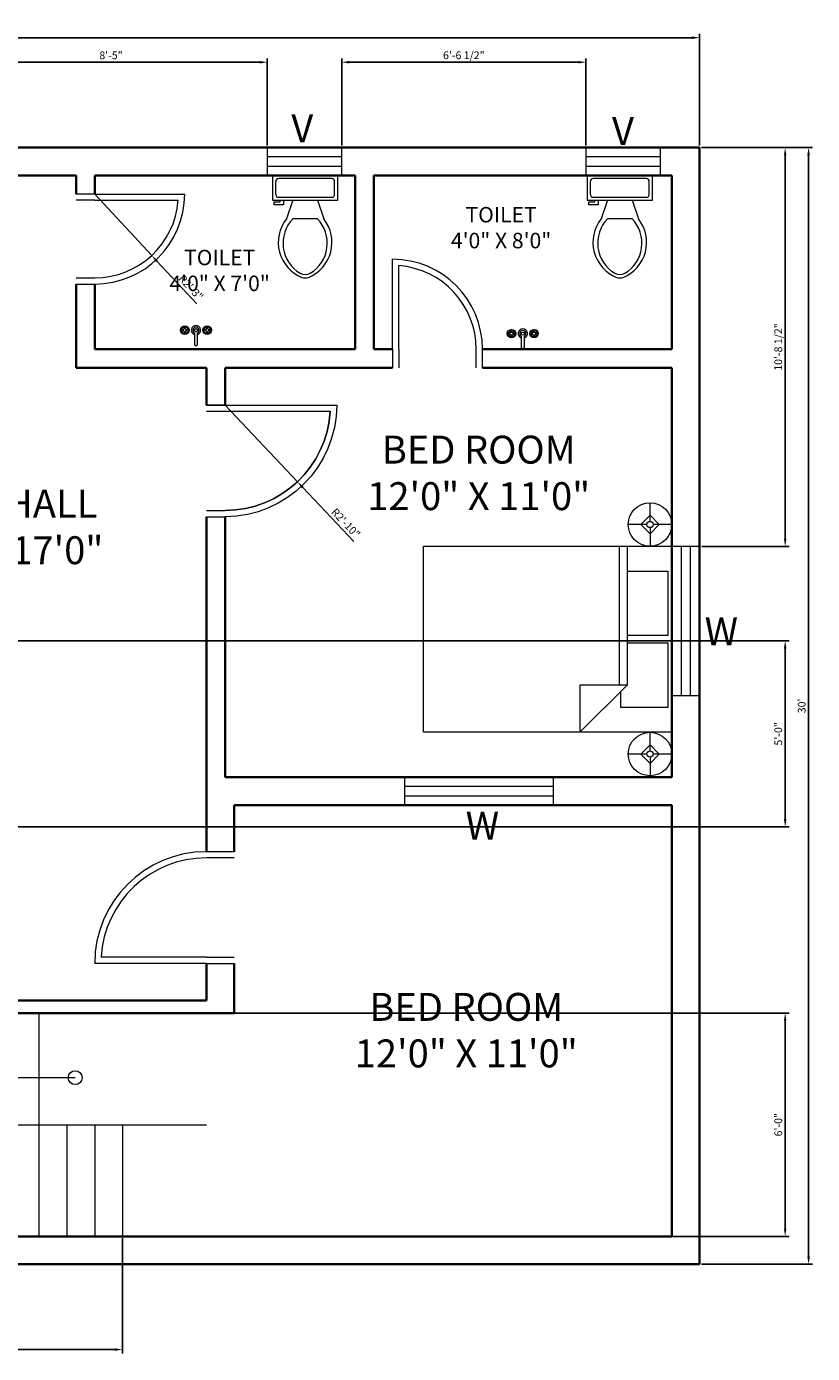
# Model space of a CAD drawing. Units: inches. Extents: x 1025 to 3479, y 1594 to 2212.
# Tile 9 of 9: x 3226 to 3479, y 1713 to 2140. Entities that reach past the tile are written whole.
import ezdxf

# ---------------------------------------------------------------- set-up
doc = ezdxf.new("R2010")
doc.units = ezdxf.units.IN
for name, color, linetype, lineweight in [('A-ANNO-DIMS', 1, 'Continuous', 18), ('A-ANNO-SYMB', 1, 'Continuous', 13), ('A-ANNO-TEXT', 7, 'Continuous', 18), ('A-AREA-IDEN', 4, 'Continuous', 18), ('A-DOOR', 4, 'Continuous', 18), ('A-FLOR-FIXT', 9, 'Continuous', 18), ('A-FLOR-STRS', 7, 'Continuous', 18), ('A-FURN', 8, 'Continuous', 13), ('A-GLAZ', 3, 'Continuous', 18), ('A-WALL', 7, 'Continuous', 35)]:
    doc.layers.add(name, color=color, linetype=linetype, lineweight=lineweight)
doc.styles.get("Standard").update_dxf_attribs({"font": 'arial.ttf'})
doc.dimstyles.new('ISO-25', dxfattribs={"dimtxt": 2.5, "dimasz": 2.5, "dimexe": 1.25, "dimexo": 0.625, "dimtad": 1, "dimdec": 0, "dimlunit": 3, "dimtxsty": 'Standard', "dimcen": 2.5, "dimadec": 0, "dimazin": 0, "dimtfac": 1, "dimtdec": 0, "dimtmove": 0, "dimatfit": 3, "dimfxl": 1, "dimarcsym": 0})

# ---------------------------------------------------------------- blocks, each defined once
blk = doc.blocks.new('*D3')
at = {"layer": 'A-ANNO-DIMS', "color": 0, "lineweight": -2, "transparency": 16777216}
for p, q in [((2962.75, 2102.12), (2962.75, 2138.14)), ((2965.25, 2136.89), (3440.25, 2136.89)), ((3442.75, 2102.12), (3442.75, 2138.14))]:
    blk.add_line(p, q, dxfattribs=at)
at = {"layer": 'A-ANNO-DIMS', "color": 0, "transparency": 16777216}
for points in [[(2965.25, 2137.31), (2965.25, 2136.48), (2962.75, 2136.89)], [(3440.25, 2137.31), (3440.25, 2136.48), (3442.75, 2136.89)]]:
    blk.add_solid(points, dxfattribs=at)
at = {"layer": 'Defpoints', "color": 0, "transparency": 16777216}
for p in [(3442.75, 2136.89), (2962.75, 2101.49), (3442.75, 2101.49)]:
    blk.add_point(p, dxfattribs=at)
at = {"layer": 'A-ANNO-DIMS', "color": 0, "transparency": 16777216, "insert": (3202.75, 2138.8), "char_height": 2.5, "attachment_point": 5}
blk.add_mtext("40'", dxfattribs=at)
blk = doc.blocks.new('*D6')
at = {"layer": 'A-ANNO-DIMS', "color": 0, "lineweight": -2, "transparency": 16777216}
for p, q in [((3443.37, 2101.49), (3479.12, 2101.49)), ((3477.87, 2098.99), (3477.87, 1743.99)), ((3443.37, 1741.49), (3479.12, 1741.49))]:
    blk.add_line(p, q, dxfattribs=at)
at = {"layer": 'A-ANNO-DIMS', "color": 0, "transparency": 16777216}
for points in [[(3477.45, 2098.99), (3478.29, 2098.99), (3477.87, 2101.49)], [(3477.45, 1743.99), (3478.29, 1743.99), (3477.87, 1741.49)]]:
    blk.add_solid(points, dxfattribs=at)
at = {"layer": 'Defpoints', "color": 0, "transparency": 16777216}
for p in [(3442.75, 2101.49), (3442.75, 1741.49), (3477.87, 1741.49)]:
    blk.add_point(p, dxfattribs=at)
at = {"layer": 'A-ANNO-DIMS', "color": 0, "transparency": 16777216, "insert": (3475.97, 1921.49), "char_height": 2.5, "attachment_point": 5, "rotation": 90}
blk.add_mtext("30'", dxfattribs=at)
blk = doc.blocks.new('Bed - Queen')
for p, q in [((0, -80.00003), (0, 0)), ((0, 0), (59.99999, 0)), ((59.99999, 0), (59.99999, -80.00003)), ((7.99999, -1.2), (28.79998, -1.2)), ((7.99999, -14.4), (7.99999, -1.2)), ((28.79998, -1.2), (28.79998, -14.4)), ((31.19999, -1.2), (51.99999, -1.2)), ((31.19999, -14.4), (31.19999, -1.2)), ((51.99999, -1.2), (51.99999, -16.4)), ((0, -14.4), (44.8, -14.4)), ((44.8, -16.8), (0, -16.8)), ((59.99999, -29.6), (44.8, -14.4)), ((44.8, -14.4), (44.8, -29.6)), ((51.99999, -16.4), (46.79936, -16.4)), ((44.8, -29.6), (59.99999, -29.6)), ((59.99999, -80.00003), (0, -80.00003))]:
    blk.add_line(p, q)
blk = doc.blocks.new('Lamp - Table')
for p, q in [((0, 7), (0, 1)), ((-1, 0), (-7, 0)), ((0, 3), (-3, 0)), ((-3, 0), (0, -3)), ((3, 0), (0, 3)), ((0, -3), (3, 0)), ((1, 0), (7, 0)), ((0, -1), (0, -7))]:
    blk.add_line(p, q)
for radius in [7, 1]:
    blk.add_circle((0, 0), radius)
blk = doc.blocks.new('Toilet - top')
for p, q in [((9.5, -6), (9.5, -2)), ((-10, -8.5), (-8, -8.5)), ((-10, -9.5), (-10, -8.5)), ((-8, -8.5), (-8, -8)), ((-7, -8), (-7, -9.5)), ((-4, -8), (-6, -14)), ((4, -8), (6, -14)), ((-7, -9.5), (-10, -9.5)), ((4, -14), (-4, -14))]:
    blk.add_line(p, q)
blk.add_lwpolyline([(10.5, -8), (10.5, 0), (-10.5, 0), (-10.5, -8)], close=True)
for points in [[(-9.5, -2), (-9.5, -6)], [(8.5, -1), (-8.5, -1)], [(-8.5, -7), (8.5, -7)]]:
    blk.add_lwpolyline(points)
for centre, radius, start, end in [((-8.62, -1.88), 0.884, 81.8699, 188.1301), ((8.62, -1.88), 0.884, 351.8699, 98.1301), ((-8.62, -6.12), 0.884, 171.8699, 278.1301), ((8.62, -6.12), 0.884, 261.8699, 8.1301), ((3.52, -21.58), 12.17, 141.4691, 247.9714), ((4.2, -21.82), 11.33, 136.3677, 238.9468), ((-3.52, -21.58), 12.17, 292.0284, 38.5307), ((-4.2, -21.82), 11.33, 301.053, 43.6321), ((0, -27.88), 4, 245.7318, 294.2682), ((0, -29), 4, 254.8605, 285.1395)]:
    blk.add_arc(centre, radius, start, end)
blk = doc.blocks.new('Faucet - Bathroom top')
for p, q in [((-4.107, 0.125), (-4.375, 0.125)), ((-3.75, 0.4788), (-3.75, 0.75)), ((-3.5, 0.482), (-3.5, 0.75)), ((-3.1461, 0.125), (-2.875, 0.125)), ((3.143, 0.125), (2.875, 0.125)), ((3.5, 0.4788), (3.5, 0.75)), ((3.75, 0.482), (3.75, 0.75)), ((4.1039, 0.125), (4.375, 0.125)), ((-4.1039, -0.125), (-4.375, -0.125)), ((-3.75, -0.4821), (-3.75, -0.75)), ((-3.5, -0.4789), (-3.5, -0.75)), ((-3.143, -0.125), (-2.875, -0.125)), ((-0.5, -0.8639), (-0.5, -4.5)), ((0.5, -4.5), (0.5, -0.8631)), ((3.1461, -0.125), (2.875, -0.125)), ((3.5, -0.4821), (3.5, -0.75)), ((3.75, -0.4789), (3.75, -0.75)), ((4.107, -0.125), (4.375, -0.125))]:
    blk.add_line(p, q)
for centre, radius in [((-3.625, 0), 1.375), ((-4.625, 0), 0.2795), ((-3.625, 0), 0.5), ((-3.625, 1), 0.2795), ((-2.625, 0), 0.2795), ((0, 0), 0.5), ((3.625, 0), 1.375), ((2.625, 0), 0.2795), ((3.625, 0), 0.5), ((3.625, 1), 0.2795), ((4.625, 0), 0.2795), ((-3.625, -1), 0.2795), ((3.625, -1), 0.2795)]:
    blk.add_circle(centre, radius)
for centre, radius, start, end in [((-3.625, 0), 1, 105.2407, 164.2093), ((-3.625, 0), 1, 16.44125, 74.07887), ((0, 0), 1.5, 289.6514, 250.3603), ((0, 0), 1, 300.3431, 239.7554), ((3.625, 0), 1, 106.12, 164.0884), ((3.625, 0), 1, 16.23422, 73.90469), ((-3.625, 0), 1, 196.2342, 253.9047), ((-3.625, 0), 1, 286.12, 344.0884), ((3.625, 0), 1, 196.4413, 254.0789), ((3.625, 0), 1, 285.2407, 344.2093), ((0, -4.5), 0.5, 180, 0)]:
    blk.add_arc(centre, radius, start, end)
blk = doc.blocks.new('WIN-48IN')
for p, q in [((0, 48), (0, 0)), ((9, 48), (0, 48)), ((3, 48), (3, 0)), ((6, 0), (6, 48)), ((9, 0), (9, 48)), ((0, 0), (9, 0))]:
    blk.add_line(p, q)
blk = doc.blocks.new('VENT-24IN')
for p, q in [((24, 9), (0, 9)), ((0, 9), (0, 0)), ((24, 0), (24, 9)), ((24, 6), (0, 6)), ((0, 3), (24, 3)), ((0, 0), (24, 0))]:
    blk.add_line(p, q)
blk = doc.blocks.new('DOOR-SWING-36IN')
for p, q in [((0, 36), (6, 36)), ((0, 34), (6, 34)), ((0, 2), (6, 2)), ((6, 0), (0, 0)), ((6, 2), (39.94, 2)), ((6, 0), (42, 0))]:
    blk.add_line(p, q)
for radius, start in [(36, 0), (34, 3.3723)]:
    blk.add_arc((6, 0), radius, start, 90)
blk = doc.blocks.new('DOOR-SWING-29IN')
for p, q in [((0, 6), (0, 35)), ((2, 6), (2, 32.93)), ((0, 6), (0, 0)), ((2, 6), (2, 0)), ((27, 0), (27, 6)), ((29, 0), (29, 6))]:
    blk.add_line(p, q)
for radius, end in [(29, 90), (27, 85.752)]:
    blk.add_arc((0, 6), radius, 0, end)
blk = doc.blocks.new('*D63')
at = {"layer": 'A-ANNO-DIMS', "color": 0, "lineweight": -2, "transparency": 16777216}
for p, q in [((3202.62, 2102.12), (3202.62, 2130.24)), ((3303.38, 2102.12), (3303.38, 2130.24)), ((3205.12, 2128.99), (3300.88, 2128.99))]:
    blk.add_line(p, q, dxfattribs=at)
at = {"layer": 'A-ANNO-DIMS', "color": 0, "transparency": 16777216}
for points in [[(3205.12, 2129.41), (3205.12, 2128.58), (3202.62, 2128.99)], [(3300.88, 2129.41), (3300.88, 2128.58), (3303.38, 2128.99)]]:
    blk.add_solid(points, dxfattribs=at)
at = {"layer": 'Defpoints', "color": 0, "transparency": 16777216}
for p in [(3303.38, 2128.99), (3202.62, 2101.49), (3303.38, 2101.49)]:
    blk.add_point(p, dxfattribs=at)
at = {"layer": 'A-ANNO-DIMS', "color": 0, "transparency": 16777216, "insert": (3253, 2130.89), "char_height": 2.5, "attachment_point": 5}
blk.add_mtext('8\'-5"', dxfattribs=at)
blk = doc.blocks.new('*D64')
at = {"layer": 'A-ANNO-DIMS', "color": 0, "lineweight": -2, "transparency": 16777216}
for p, q in [((3327.38, 2102.12), (3327.38, 2130.24)), ((3406.1, 2102.12), (3406.1, 2130.24)), ((3329.88, 2128.99), (3403.6, 2128.99))]:
    blk.add_line(p, q, dxfattribs=at)
at = {"layer": 'A-ANNO-DIMS', "color": 0, "transparency": 16777216}
for points in [[(3329.88, 2129.41), (3329.88, 2128.58), (3327.38, 2128.99)], [(3403.6, 2129.41), (3403.6, 2128.58), (3406.1, 2128.99)]]:
    blk.add_solid(points, dxfattribs=at)
at = {"layer": 'Defpoints', "color": 0, "transparency": 16777216}
for p in [(3406.1, 2128.99), (3327.38, 2101.49), (3406.1, 2101.49)]:
    blk.add_point(p, dxfattribs=at)
at = {"layer": 'A-ANNO-DIMS', "color": 0, "transparency": 16777216, "insert": (3366.74, 2130.91), "char_height": 2.5, "attachment_point": 5}
blk.add_mtext('6\'-6 1/2"', dxfattribs=at)
blk = doc.blocks.new('*D76')
at = {"layer": 'A-ANNO-DIMS', "color": 0, "lineweight": -2, "transparency": 16777216}
for p, q in [((3443.37, 2101.49), (3471.57, 2101.49)), ((3470.32, 2098.99), (3470.32, 1975.38)), ((3443.45, 1972.88), (3471.57, 1972.88))]:
    blk.add_line(p, q, dxfattribs=at)
at = {"layer": 'A-ANNO-DIMS', "color": 0, "transparency": 16777216}
for points in [[(3469.91, 2098.99), (3470.74, 2098.99), (3470.32, 2101.49)], [(3469.91, 1975.38), (3470.74, 1975.38), (3470.32, 1972.88)]]:
    blk.add_solid(points, dxfattribs=at)
at = {"layer": 'Defpoints', "color": 0, "transparency": 16777216}
for p in [(3442.75, 2101.49), (3442.82, 1972.88), (3470.32, 1972.88)]:
    blk.add_point(p, dxfattribs=at)
at = {"layer": 'A-ANNO-DIMS', "color": 0, "transparency": 16777216, "insert": (3468.41, 2037.19), "char_height": 2.5, "attachment_point": 5, "rotation": 90}
blk.add_mtext('10\'-8 1/2"', dxfattribs=at)
blk = doc.blocks.new('*D82')
at = {"layer": 'A-ANNO-DIMS', "color": 0, "lineweight": -2, "transparency": 16777216}
for p, q in [((3121.75, 1749.87), (3121.75, 1712.74)), ((3256.75, 1749.87), (3256.75, 1712.74)), ((3124.25, 1713.99), (3254.25, 1713.99))]:
    blk.add_line(p, q, dxfattribs=at)
at = {"layer": 'A-ANNO-DIMS', "color": 0, "transparency": 16777216}
for points in [[(3124.25, 1714.41), (3124.25, 1713.58), (3121.75, 1713.99)], [(3254.25, 1714.41), (3254.25, 1713.58), (3256.75, 1713.99)]]:
    blk.add_solid(points, dxfattribs=at)
at = {"layer": 'Defpoints', "color": 0, "transparency": 16777216}
for p in [(3121.75, 1750.49), (3256.75, 1750.49), (3256.75, 1713.99)]:
    blk.add_point(p, dxfattribs=at)
at = {"layer": 'A-ANNO-DIMS', "color": 0, "transparency": 16777216, "insert": (3189.25, 1715.89), "char_height": 2.5, "attachment_point": 5}
blk.add_mtext('11\'-3"', dxfattribs=at)
blk = doc.blocks.new('*D83')
at = {"layer": 'A-ANNO-DIMS', "color": 0, "lineweight": -2, "transparency": 16777216}
for p, q in [((3284.37, 1822.49), (3471.57, 1822.49)), ((3470.32, 1752.99), (3470.32, 1819.99)), ((3257.37, 1750.49), (3471.57, 1750.49))]:
    blk.add_line(p, q, dxfattribs=at)
at = {"layer": 'A-ANNO-DIMS', "color": 0, "transparency": 16777216}
for points in [[(3469.91, 1819.99), (3470.74, 1819.99), (3470.32, 1822.49)], [(3469.91, 1752.99), (3470.74, 1752.99), (3470.32, 1750.49)]]:
    blk.add_solid(points, dxfattribs=at)
at = {"layer": 'Defpoints', "color": 0, "transparency": 16777216}
for p in [(3283.75, 1822.49), (3470.32, 1822.49), (3256.75, 1750.49)]:
    blk.add_point(p, dxfattribs=at)
at = {"layer": 'A-ANNO-DIMS', "color": 0, "transparency": 16777216, "insert": (3468.42, 1786.49), "char_height": 2.5, "attachment_point": 5, "rotation": 90}
blk.add_mtext('6\'-0"', dxfattribs=at)
blk = doc.blocks.new('*D85')
at = {"layer": 'A-ANNO-DIMS', "color": 0, "lineweight": -2, "transparency": 16777216}
for p, q in [((3116.37, 1942.49), (3471.57, 1942.49)), ((3470.32, 1884.99), (3470.32, 1939.99)), ((3116.37, 1882.49), (3471.57, 1882.49))]:
    blk.add_line(p, q, dxfattribs=at)
at = {"layer": 'A-ANNO-DIMS', "color": 0, "transparency": 16777216}
for points in [[(3469.91, 1939.99), (3470.74, 1939.99), (3470.32, 1942.49)], [(3469.91, 1884.99), (3470.74, 1884.99), (3470.32, 1882.49)]]:
    blk.add_solid(points, dxfattribs=at)
at = {"layer": 'Defpoints', "color": 0, "transparency": 16777216}
for p in [(3115.75, 1942.49), (3470.32, 1942.49), (3115.75, 1882.49)]:
    blk.add_point(p, dxfattribs=at)
at = {"layer": 'A-ANNO-DIMS', "color": 0, "transparency": 16777216, "insert": (3468.42, 1912.49), "char_height": 2.5, "attachment_point": 5, "rotation": 90}
blk.add_mtext('5\'-0"', dxfattribs=at)
blk = doc.blocks.new('*D92')
at = {"layer": 'A-ANNO-DIMS', "color": 0, "lineweight": -2, "transparency": 16777216}
for p, q in [((3289.75, 2018.49), (3313.07, 1993.75)), ((3331.26, 1974.46), (3314.79, 1991.93))]:
    blk.add_line(p, q, dxfattribs=at)
at = {"layer": 'A-ANNO-DIMS', "color": 0, "transparency": 16777216}
blk.add_solid([(3315.09, 1992.22), (3314.48, 1991.65), (3313.07, 1993.75)], dxfattribs=at)
at = {"layer": 'Defpoints', "color": 0, "transparency": 16777216}
for p in [(3289.75, 2018.49), (3313.07, 1993.75)]:
    blk.add_point(p, dxfattribs=at)
at = {"layer": 'A-ANNO-DIMS', "color": 0, "transparency": 16777216, "insert": (3328.45, 1980.21), "char_height": 2.5, "attachment_point": 5, "rotation": 313.3133}
blk.add_mtext('R2\'-10"', dxfattribs=at)
blk = doc.blocks.new('*D99')
at = {"layer": 'A-ANNO-DIMS', "color": 0, "lineweight": -2, "transparency": 16777216}
for p, q in [((3247.75, 2086.49), (3266.12, 2066.71)), ((3280.64, 2051.06), (3267.82, 2064.87))]:
    blk.add_line(p, q, dxfattribs=at)
at = {"layer": 'A-ANNO-DIMS', "color": 0, "transparency": 16777216}
blk.add_solid([(3268.12, 2065.16), (3267.51, 2064.59), (3266.12, 2066.71)], dxfattribs=at)
at = {"layer": 'Defpoints', "color": 0, "transparency": 16777216}
for p in [(3247.75, 2086.49), (3266.12, 2066.71)]:
    blk.add_point(p, dxfattribs=at)
at = {"layer": 'A-ANNO-DIMS', "color": 0, "transparency": 16777216, "insert": (3278.53, 2056.13), "char_height": 2.5, "attachment_point": 5, "rotation": 312.8758}
blk.add_mtext('R2\'-3"', dxfattribs=at)

msp = doc.modelspace()

# ---------------------------------------------------------------- linework, layer by layer
at = {"layer": 'A-ANNO-SYMB'}
msp.add_line((3241.46, 1801.64), (3139.54, 1801.64), dxfattribs=at)
msp.add_circle((3241.46, 1801.64), 2.24, dxfattribs=at)
at = {"layer": 'A-DOOR'}
for p, q in [((3276.68, 2084.49), (3276.75, 2084.49)), ((3345.75, 2065.42), (3345.75, 2065.49)), ((3283.75, 2018.49), (3289.75, 2018.49)), ((3325.69, 2016.49), (3325.75, 2016.49)), ((3292.75, 1874.49), (3283.75, 1874.49)), ((3292.75, 1872.49), (3283.75, 1872.49)), ((3247.8, 1840.49), (3247.75, 1840.49)), ((3283.75, 1840.49), (3249.81, 1840.49)), ((3283.75, 1840.49), (3292.75, 1840.49)), ((3283.75, 1838.49), (3247.75, 1838.49)), ((3283.75, 1838.49), (3292.75, 1838.49))]:
    msp.add_line(p, q, dxfattribs=at)
for centre, radius, start, end in [((3289.75, 2018.49), 34, 270, 356.6277), ((3283.75, 1838.49), 36, 90, 180), ((3283.75, 1838.49), 34, 90, 176.6277)]:
    msp.add_arc(centre, radius, start, end, dxfattribs=at)
at = {"layer": 'A-FLOR-STRS'}
for p, q in [((3229.75, 1822.49), (3229.75, 1750.49)), ((3121.75, 1786.49), (3283.75, 1786.49)), ((3238.75, 1786.49), (3238.75, 1750.49)), ((3247.75, 1786.49), (3247.75, 1750.49)), ((3256.75, 1786.49), (3256.75, 1750.49))]:
    msp.add_line(p, q, dxfattribs=at)
at = {"layer": 'A-WALL'}
for p, q in [((2962.75, 2101.49), (3442.75, 2101.49)), ((3442.75, 2101.49), (3442.75, 1741.49)), ((3211.75, 2092.49), (3241.75, 2092.49)), ((3241.75, 2092.49), (3241.75, 2086.49)), ((3247.75, 2092.49), (3247.75, 2086.49)), ((3247.75, 2092.49), (3283.75, 2092.49)), ((3247.75, 2092.49), (3247.75, 2086.49)), ((3283.75, 2092.49), (3289.75, 2092.49)), ((3289.75, 2092.49), (3331.75, 2092.49)), ((3331.75, 2092.49), (3331.75, 2036.49)), ((3337.75, 2092.49), (3337.75, 2036.49)), ((3337.75, 2092.49), (3433.75, 2092.49)), ((3433.75, 2092.49), (3433.75, 2036.49)), ((3241.75, 2057.49), (3241.75, 2036.49)), ((3247.75, 2057.49), (3247.75, 2036.49)), ((3241.75, 2036.49), (3241.75, 2030.49)), ((3247.75, 2036.49), (3283.75, 2036.49)), ((3289.75, 2036.49), (3282.72, 2036.49)), ((3289.75, 2036.49), (3331.75, 2036.49)), ((3337.75, 2036.49), (3343.75, 2036.49)), ((3337.75, 2036.49), (3343.75, 2036.49)), ((3337.75, 2036.49), (3343.75, 2036.49)), ((3372.75, 2036.49), (3433.75, 2036.49)), ((3241.75, 2030.49), (3283.75, 2030.49)), ((3283.75, 2030.49), (3283.75, 2018.49)), ((3283.75, 2030.49), (3283.75, 2018.49)), ((3289.75, 2030.49), (3289.75, 2018.49)), ((3289.75, 2030.49), (3343.75, 2030.49)), ((3372.75, 2030.49), (3433.75, 2030.49)), ((3433.75, 2030.49), (3433.75, 1898.49)), ((3283.75, 1982.49), (3283.75, 1874.49)), ((3289.75, 1982.49), (3289.75, 1898.49)), ((3289.75, 1898.49), (3433.75, 1898.49)), ((3292.75, 1889.49), (3433.75, 1889.49)), ((3292.75, 1889.49), (3292.75, 1874.49)), ((3433.75, 1889.49), (3433.75, 1826.49)), ((3283.75, 1826.49), (3283.75, 1838.49)), ((3283.75, 1838.49), (3283.75, 1826.49)), ((3292.75, 1838.49), (3292.75, 1826.49)), ((3121.75, 1826.49), (3283.75, 1826.49)), ((3121.75, 1822.49), (3283.75, 1822.49)), ((3283.75, 1822.49), (3292.75, 1822.49)), ((3292.75, 1826.49), (3292.75, 1822.49)), ((3433.75, 1826.49), (3433.75, 1813.62)), ((3433.75, 1817.49), (3433.75, 1750.49)), ((3433.75, 1750.49), (3121.75, 1750.49)), ((3442.75, 1741.49), (2962.75, 1741.49))]:
    msp.add_line(p, q, dxfattribs=at)

# ---------------------------------------------------------------- block references
at = {"layer": 'A-DOOR', "rotation": 270.0000000000037}
msp.add_blockref('DOOR-SWING-29IN', (3241.75, 2086.49), dxfattribs=at)
at = {"layer": 'A-DOOR'}
msp.add_blockref('DOOR-SWING-29IN', (3343.75, 2030.49), dxfattribs=at)
at = {"layer": 'A-DOOR', "extrusion": (0, 0, -1), "zscale": -1, "rotation": 180}
msp.add_blockref('DOOR-SWING-36IN', (-3283.75, 2018.49), dxfattribs=at)
at = {"layer": 'A-FLOR-FIXT'}
for name, p in [('Toilet - top', (3315.58, 2092.49)), ('Toilet - top', (3417.01, 2092.49)), ('Faucet - Bathroom top', (3280.4, 2042.62)), ('Faucet - Bathroom top', (3385.74, 2041.51))]:
    msp.add_blockref(name, p, dxfattribs=at)
at = {"layer": 'A-FURN', "rotation": 270}
for name, p in [('Lamp - Table', (3426.75, 1979.98)), ('Bed - Queen', (3433.75, 1972.98)), ('Lamp - Table', (3426.75, 1905.98))]:
    msp.add_blockref(name, p, dxfattribs=at)
at = {"layer": 'A-GLAZ'}
for name, p in [('VENT-24IN', (3303.38, 2092.49)), ('VENT-24IN', (3406.1, 2092.49)), ('WIN-48IN', (3433.82, 1924.88))]:
    msp.add_blockref(name, p, dxfattribs=at)
at = {"layer": 'A-GLAZ', "rotation": 270.0000000000016}
msp.add_blockref('WIN-48IN', (3347.6, 1898.49), dxfattribs=at)

# ---------------------------------------------------------------- texts
at = {"layer": 'A-ANNO-TEXT', "char_height": 9, "attachment_point": 1}
for s, width, insert in [('\\pxqc;{V}', 7.8272, (3310.74, 2112.19)), ('\\pxqc;{V}', 7.8272, (3414.12, 2111.3)), ('\\pxqc;W', 15.8719, (3441.8, 1950.03)), ('\\pxqc;W', 15.8719, (3364.79, 1887.37))]:
    msp.add_mtext_dynamic_manual_height_columns(s, width=width, gutter_width=12.5, heights=[0], dxfattribs=dict(at, insert=insert))
at = {"layer": 'A-AREA-IDEN', "attachment_point": 1}
for s, width, insert, char_height in [('\\pxqc;TOILET \\P4\'0" X 8\'0"', 51.1118, (3353.19, 2082.34), 5), ('\\pxqc;TOILET \\P4\'0" X 7\'0" ', 51.1118, (3262.47, 2068.54), 5), ('\\pxqc;BED ROOM \\P12\'0" X 11\'0"', 93.2353, (3324.92, 2008.61), 9), ('\\pxqc;LIVING HALL \\P13\'0"  X 17\'0"', 93.2353, (3166.61, 1991.18), 9), ('\\pxqc;BED ROOM \\P12\'0" X 11\'0"', 93.2353, (3320.9, 1828.97), 9)]:
    msp.add_mtext_dynamic_manual_height_columns(s, width=width, gutter_width=12.5, heights=[0], dxfattribs=dict(at, insert=insert, char_height=char_height))

# ---------------------------------------------------------------- dimensions: what is measured, and where the dimension line sits
at = {"layer": 'A-ANNO-DIMS'}
for base, p1, p2, override, picture, middle in [((3442.75, 2136.89), (2962.75, 2101.49), (3442.75, 2101.49), {"dimclrd": 0, "dimclre": 0, "dimclrt": 0}, '*D3', (3202.75, 2138.8)), ((3406.1, 2128.99), (3327.38, 2101.49), (3406.1, 2101.49), {"dimdec": 1, "dimlfac": 1, "dimrnd": 0, "dimzin": 1, "dimdsep": 46, "dimlunit": 4, "dimfrac": 2}, '*D64', (3366.74, 2130.91)), ((3303.38, 2128.99), (3202.62, 2101.49), (3303.38, 2101.49), {"dimdec": 1, "dimlfac": 1, "dimrnd": 0, "dimzin": 1, "dimdsep": 46, "dimlunit": 4, "dimfrac": 2}, '*D63', (3253, 2130.89)), ((3256.75, 1713.99), (3121.75, 1750.49), (3256.75, 1750.49), {"dimdec": 1, "dimlfac": 1, "dimrnd": 0, "dimzin": 1, "dimdsep": 46, "dimlunit": 4, "dimfrac": 2}, '*D82', (3189.25, 1715.89))]:
    dim = msp.add_linear_dim(base=base, p1=p1, p2=p2, dimstyle='ISO-25', override=override, dxfattribs=at)
    dim.commit()
    dim.dimension.update_dxf_attribs({"geometry": picture, "text_midpoint": middle})
for base, p1, p2, override, picture, middle in [((3477.87, 1741.49), (3442.75, 2101.49), (3442.75, 1741.49), {"dimclrd": 0, "dimclre": 0, "dimclrt": 0}, '*D6', (3475.97, 1921.49)), ((3470.32, 1972.88), (3442.75, 2101.49), (3442.82, 1972.88), {"dimdec": 1, "dimlfac": 1, "dimrnd": 0, "dimzin": 1, "dimdsep": 46, "dimlunit": 4, "dimfrac": 2}, '*D76', (3468.41, 2037.19)), ((3470.32, 1942.49), (3115.75, 1882.49), (3115.75, 1942.49), {"dimdec": 1, "dimlfac": 1, "dimrnd": 0, "dimzin": 1, "dimdsep": 46, "dimlunit": 4, "dimfrac": 2}, '*D85', (3468.42, 1912.49)), ((3470.32, 1822.49), (3256.75, 1750.49), (3283.75, 1822.49), {"dimdec": 1, "dimlfac": 1, "dimrnd": 0, "dimzin": 1, "dimdsep": 46, "dimlunit": 4, "dimfrac": 2}, '*D83', (3468.42, 1786.49))]:
    dim = msp.add_linear_dim(base=base, p1=p1, p2=p2, angle=90, dimstyle='ISO-25', override=override, dxfattribs=at)
    dim.commit()
    dim.dimension.update_dxf_attribs({"geometry": picture, "text_midpoint": middle})
for center, mpoint, picture, middle in [((3247.75, 2086.49), (3266.12, 2066.71), '*D99', (3277.14, 2054.83)), ((3289.75, 2018.49), (3313.07, 1993.75), '*D92', (3327.06, 1978.91))]:
    dim = msp.add_radius_dim(center=center, mpoint=mpoint, dimstyle='ISO-25', override={"dimdec": 1, "dimlfac": 1, "dimrnd": 0, "dimzin": 1, "dimdsep": 46, "dimlunit": 4, "dimfrac": 2}, dxfattribs=at)
    dim.commit()
    dim.dimension.update_dxf_attribs({"geometry": picture, "text_midpoint": middle, "dimtype": 164})

doc.saveas('drawing.dxf')
